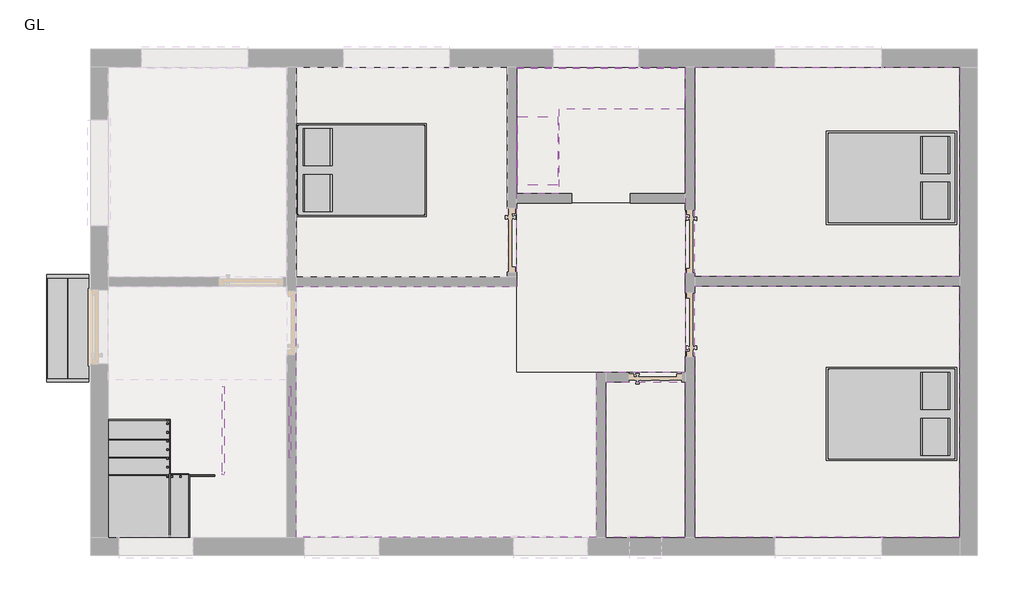
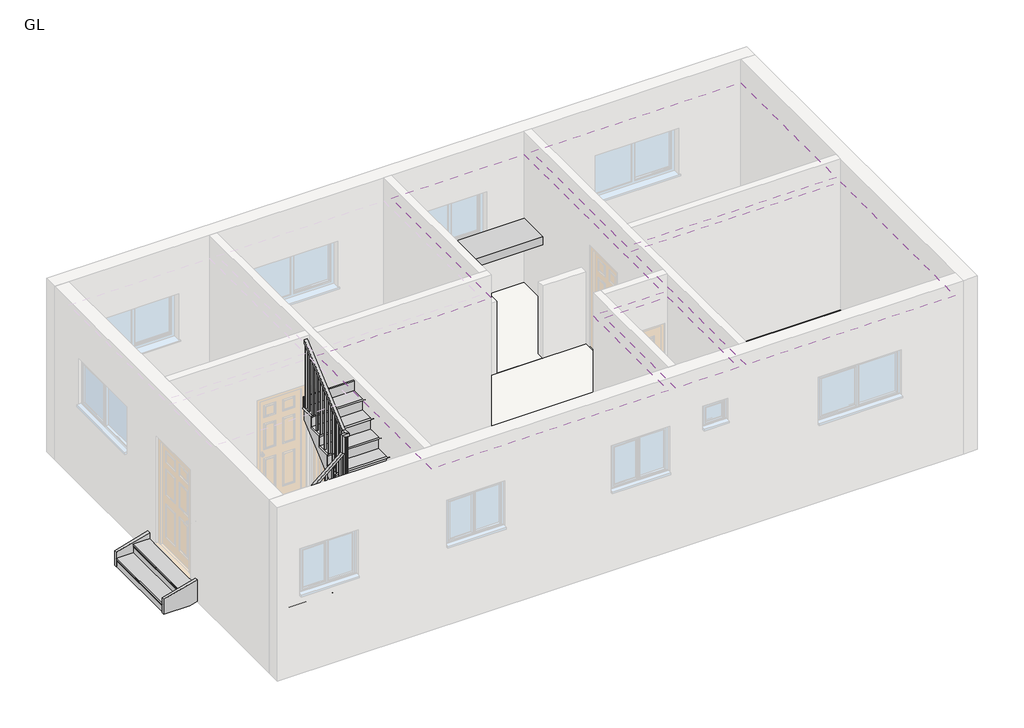
# One storey, part 2 of 2: 7 members, 5 slabs, 4 coverings, 3 furniture elements, 2 proxies, 2 stair flights, 1 railing.
"""IFC4 building model written with IfcOpenShell, lengths in millimetres."""

from ifc_helpers import new_model, si_unit, frame, origin, place, context, project, spatial, polyline, outline, extrude, faceted_brep, transform, mapped, element, save
from components import proxy_0915_x_500_mm_892363c5, furniture_bed_1_1346x1880x355mm_double_93dec6ea, wood_steps_w_30mm_tread_25mm_nosing_19mm_riser_e02fc27e, wood_steps_w_50mm_tread_10mm_nosing_13mm_riser_13d2c295

model = new_model("IFC4")

# Units and contexts
model_context = context("Model", 3, world=origin())
ifc_project = project(units=[si_unit("LENGTHUNIT", "METRE", prefix="MILLI")], contexts=[model_context])

# Site, building, storey
site = spatial("IfcSite", under=ifc_project)
building = spatial("IfcBuilding", under=site)
storey = spatial("IfcBuildingStorey", under=building, Name="GL", Elevation=0.0)

# Proxies
placement = place(None, origin())
proxy_0915_x_500_mm_shape = proxy_0915_x_500_mm_892363c5(model_context)
element("IfcBuildingElementProxy", 1, Name="0915 x 500 mm", ObjectType="0915 x 500 mm", at=placement, inside=storey, context=model_context, shape_type="MappedRepresentation", body=[
    mapped(proxy_0915_x_500_mm_shape, transform((1909.0522582, 5351.5962501, 467.868), x_axis=(0.0, 1.0, 0.0), y_axis=(-1.0, 0.0, 0.0), z_axis=(0.0, 0.0, 1.0))),
])
element("IfcBuildingElementProxy", 2, Name="Generic Models 1 : Generic Models 1", ObjectType="Generic Models 1 : Generic Models 1", at=placement, inside=storey, context=model_context, shape_type="SweptSolid", body=[
    extrude(outline(polyline([(2213.8522582, 4735.0444495), (1604.2522582, 4735.0444495), (1604.2522582, 6545.3962501), (4029.9522582, 6545.3962501), (4029.9522582, 5954.2444495), (2213.8522582, 5954.2444495), (2213.8522582, 4735.0444495)])), frame((0.0, 0.0, 1219.2), z_axis=(0.0, 0.0, 1.0), x_axis=(1.0, 0.0, 0.0)), (0.0, 0.0, 1.0), 152.4),
])

# Coverings
element("IfcCovering", 3, ObjectType="Plain", at=placement, inside=storey, context=model_context, shape_type="SweptSolid", body=[
    extrude(outline(polyline([(1604.2522582, 6562.8522428), (4033.9673421, 6562.8522428), (4033.9673421, 2153.4122428), (2751.2673421, 2153.4122428), (2751.2673421, -234.1877572), (-1580.4996772, -234.1877572), (-1580.4996772, 3389.7573971), (1604.2522582, 3389.7573971), (1604.2522582, 6562.8522428)])), frame((0.0, 0.0, 2600.0), z_axis=(0.0, 0.0, 1.0), x_axis=(1.0, 0.0, 0.0)), (0.0, 0.0, 1.0), 57.0),
])
element("IfcCovering", 4, ObjectType="Plain", at=placement, inside=storey, context=model_context, shape_type="SweptSolid", body=[
    extrude(outline(polyline([(4171.1273421, 6562.8522428), (7994.8922582, 6562.8522428), (7994.8922582, 3534.6060854), (4171.1273421, 3534.6060854), (4171.1273421, 6562.8522428)])), frame((0.0, 0.0, 2600.0), z_axis=(0.0, 0.0, 1.0), x_axis=(1.0, 0.0, 0.0)), (0.0, 0.0, 1.0), 57.0),
])
element("IfcCovering", 5, ObjectType="Plain", at=placement, inside=storey, context=model_context, shape_type="SweptSolid", body=[
    extrude(outline(polyline([(4171.1273421, 3397.4460854), (7994.8922582, 3397.4460854), (7994.8922582, -234.1877572), (4171.1273421, -234.1877572), (4171.1273421, 3397.4460854)])), frame((0.0, 0.0, 2600.0), z_axis=(0.0, 0.0, 1.0), x_axis=(1.0, 0.0, 0.0)), (0.0, 0.0, 1.0), 57.0),
])
element("IfcCovering", 6, ObjectType="Plain", at=placement, inside=storey, context=model_context, shape_type="SweptSolid", body=[
    extrude(outline(polyline([(4033.9673421, 2016.2522428), (4033.9673421, -234.1877572), (2888.4273421, -234.1877572), (2888.4273421, 2016.2522428), (4033.9673421, 2016.2522428)])), frame((0.0, 0.0, 2600.0), z_axis=(0.0, 0.0, 1.0), x_axis=(1.0, 0.0, 0.0)), (0.0, 0.0, 1.0), 57.0),
])

# Furniture
furniture_bed_1_1346x1880x355mm_double_shape = furniture_bed_1_1346x1880x355mm_double_93dec6ea(model_context)
element("IfcFurniture", 7, ObjectType="Furniture_Bed_1 : 1346x1880x355mm-Double", at=placement, inside=storey, context=model_context, shape_type="MappedRepresentation", body=[
    mapped(furniture_bed_1_1346x1880x355mm_double_shape, transform((7249.2052658, 1890.4847018, 124.968), x_axis=(0.0, -1.0, 0.0), y_axis=(1.0, 0.0, 0.0), z_axis=(0.0, 0.0, 1.0))),
])
element("IfcFurniture", 8, ObjectType="Furniture_Bed_1 : 1346x1880x355mm-Double", at=placement, inside=storey, context=model_context, shape_type="MappedRepresentation", body=[
    mapped(furniture_bed_1_1346x1880x355mm_double_shape, transform((7249.2052658, 5301.0698561, 124.968), x_axis=(0.0, -1.0, 0.0), y_axis=(1.0, 0.0, 0.0), z_axis=(0.0, 0.0, 1.0))),
])
element("IfcFurniture", 9, ObjectType="Furniture_Bed_1 : 1346x1880x355mm-Double", at=placement, inside=storey, context=model_context, shape_type="MappedRepresentation", body=[
    mapped(furniture_bed_1_1346x1880x355mm_double_shape, transform((-874.9291854, 4735.0444495, 124.968), x_axis=(0.0, 1.0, 0.0), y_axis=(-1.0, 0.0, 0.0), z_axis=(0.0, 0.0, 1.0))),
])

# Members
element("IfcMember", 10, ObjectType="Stringer-50mm_Width", at=placement, inside=storey, context=model_context, shape_type="SweptSolid", body=[
    extrude(outline(polyline([(-19.9608904, -5182.6277418), (-304.8, -5182.6277418), (-304.8, -4709.8631575), (-267.1702607, -4573.0277418), (147.6791096, -4573.0277418), (-19.9608904, -5182.6277418)])), frame((0.0, 3514.2173971, 0.0), z_axis=(0.0, 1.0, 0.0), x_axis=(0.0, 0.0, 1.0)), (0.0, 0.0, 1.0), 50.0),
])
element("IfcMember", 11, ObjectType="Stringer-50mm_Width", at=placement, inside=storey, context=model_context, shape_type="SweptSolid", body=[
    extrude(outline(polyline([(-19.9608904, -5182.6277418), (-304.8, -5182.6277418), (-304.8, -4709.8631575), (-267.1702607, -4573.0277418), (147.6791096, -4573.0277418), (-19.9608904, -5182.6277418)])), frame((0.0, 2010.6912809, 0.0), z_axis=(0.0, 1.0, 0.0), x_axis=(0.0, 0.0, 1.0)), (0.0, 0.0, 1.0), 50.0),
])
element("IfcMember", 12, ObjectType="Stringer-50mm_Width", at=placement, inside=storey, context=model_context, shape_type="Brep", body=[
    faceted_brep([(-3412.2477418, 1428.6922428, 0.0), (-3412.2477418, 1164.46764, 0.0), (-3437.2477418, 1164.46764, 0.0), (-3437.2477418, 1428.6922428, 0.0), (-3412.2477418, 1428.6922428, 168.645103), (-3412.2477418, 1406.4448629, 187.7142857), (-3412.2477418, 1137.5414829, 187.7142857), (-3412.2477418, 1137.5414829, 405.4285714), (-3412.2477418, 883.5414829, 405.4285714), (-3412.2477418, 883.5414829, 623.1428571), (-3412.2477418, 673.5414829, 623.1428571), (-3412.2477418, 673.5414829, 420.793849), (-3412.2477418, 883.5414829, 240.793849), (-3412.2477418, 1137.5414829, 23.0795633), (-3437.2477418, 673.5414829, 420.793849), (-3437.2477418, 673.5414829, 623.1428571), (-3437.2477418, 1428.6922428, 168.645103), (-3437.2477418, 1137.5414829, 187.7142857), (-3437.2477418, 1406.4448629, 187.7142857), (-3437.2477418, 883.5414829, 623.1428571), (-3437.2477418, 883.5414829, 405.4285714), (-3437.2477418, 1137.5414829, 405.4285714)], [[[0, 1, 2, 3]], [[4, 5, 6, 7, 8, 9, 10, 11, 12, 13, 1, 0]], [[14, 11, 10, 15]], [[11, 14, 2, 1, 13, 12]], [[16, 4, 0, 3]], [[17, 6, 5, 18]], [[18, 16, 3, 2, 14, 15, 19, 20, 21, 17]], [[16, 18, 5, 4]], [[6, 17, 21, 7]], [[7, 21, 20, 8]], [[8, 20, 19, 9]], [[9, 19, 15, 10]]]),
])
element("IfcMember", 13, ObjectType="Stringer-50mm_Width", at=placement, inside=storey, context=model_context, shape_type="Brep", body=[
    faceted_brep([(-3437.2477418, 673.5414829, 618.064712), (-3437.2477418, 673.5414829, 623.1428571), (-3431.2775454, 673.5414829, 623.1428571), (-3437.2477418, 648.5414829, 618.064712), (-3431.2775454, 648.5414829, 623.1428571), (-3437.2477418, 648.5414829, 623.1428571)], [[[0, 1, 2]], [[3, 0, 2, 4]], [[5, 3, 4]], [[0, 3, 5, 1]], [[2, 1, 5, 4]]]),
    faceted_brep([(-2644.3706787, 673.5414829, 1494.0), (-2644.3706787, 673.5414829, 1292.4721338), (-2854.3706787, 673.5414829, 1113.849791), (-3114.2477418, 673.5414829, 892.8028869), (-3368.2477418, 673.5414829, 676.7549104), (-3412.2477418, 673.5414829, 639.3292766), (-3412.2477418, 673.5414829, 840.8571429), (-3368.2477418, 673.5414829, 840.8571429), (-3368.2477418, 673.5414829, 1058.5714286), (-3114.2477418, 673.5414829, 1058.5714286), (-3114.2477418, 673.5414829, 1276.2857143), (-2854.3706787, 673.5414829, 1276.2857143), (-2854.3706787, 673.5414829, 1494.0), (-2644.3706787, 648.5414829, 1292.4721338), (-3412.2477418, 648.5414829, 639.3292766), (-2644.3706787, 648.5414829, 1494.0), (-2854.3706787, 648.5414829, 1494.0), (-2854.3706787, 648.5414829, 1276.2857143), (-3114.2477418, 648.5414829, 1276.2857143), (-3114.2477418, 648.5414829, 1058.5714286), (-3368.2477418, 648.5414829, 1058.5714286), (-3368.2477418, 648.5414829, 840.8571429), (-3412.2477418, 648.5414829, 840.8571429)], [[[0, 1, 2, 3, 4, 5, 6, 7, 8, 9, 10, 11, 12]], [[1, 13, 14, 5, 4, 3, 2]], [[14, 13, 15, 16, 17, 18, 19, 20, 21, 22]], [[13, 1, 0, 15]], [[10, 18, 17, 11]], [[6, 22, 21, 7]], [[22, 6, 5, 14]], [[8, 20, 19, 9]], [[7, 21, 20, 8]], [[18, 10, 9, 19]], [[12, 16, 15, 0]], [[11, 17, 16, 12]]]),
])
element("IfcMember", 14, ObjectType="Stringer-50mm_Width", at=placement, inside=storey, context=model_context, shape_type="Brep", body=[
    faceted_brep([(-2619.3706787, 1948.6214829, 2602.2909918), (-2644.3706787, 1948.6214829, 2602.2909918), (-2644.3706787, 1948.6214829, 2800.2857143), (-2619.3706787, 1948.6214829, 2800.2857143), (-2644.3706787, 1733.5414829, 2417.9367061), (-2644.3706787, 1479.5414829, 2200.2224204), (-2644.3706787, 1225.5414829, 1982.5081347), (-2644.3706787, 971.5414829, 1764.793849), (-2644.3706787, 717.5414829, 1547.0795633), (-2644.3706787, 673.5414829, 1509.3652775), (-2644.3706787, 673.5414829, 1711.7142857), (-2644.3706787, 717.5414829, 1711.7142857), (-2644.3706787, 717.5414829, 1929.4285714), (-2644.3706787, 971.5414829, 1929.4285714), (-2644.3706787, 971.5414829, 2147.1428571), (-2644.3706787, 1225.5414829, 2147.1428571), (-2644.3706787, 1225.5414829, 2364.8571429), (-2644.3706787, 1479.5414829, 2364.8571429), (-2644.3706787, 1479.5414829, 2582.5714286), (-2644.3706787, 1733.5414829, 2582.5714286), (-2644.3706787, 1733.5414829, 2800.2857143), (-2619.3706787, 673.5414829, 1509.3652775), (-2619.3706787, 1733.5414829, 2800.2857143), (-2619.3706787, 1733.5414829, 2582.5714286), (-2619.3706787, 1479.5414829, 2582.5714286), (-2619.3706787, 1479.5414829, 2364.8571429), (-2619.3706787, 1225.5414829, 2364.8571429), (-2619.3706787, 1225.5414829, 2147.1428571), (-2619.3706787, 971.5414829, 2147.1428571), (-2619.3706787, 971.5414829, 1929.4285714), (-2619.3706787, 717.5414829, 1929.4285714), (-2619.3706787, 717.5414829, 1711.7142857), (-2619.3706787, 673.5414829, 1711.7142857)], [[[0, 1, 2, 3]], [[2, 1, 4, 5, 6, 7, 8, 9, 10, 11, 12, 13, 14, 15, 16, 17, 18, 19, 20]], [[1, 0, 21, 9, 8, 7, 6, 5, 4]], [[0, 3, 22, 23, 24, 25, 26, 27, 28, 29, 30, 31, 32, 21]], [[10, 32, 31, 11]], [[32, 10, 9, 21]], [[12, 30, 29, 13]], [[11, 31, 30, 12]], [[14, 28, 27, 15]], [[13, 29, 28, 14]], [[16, 26, 25, 17]], [[15, 27, 26, 16]], [[18, 24, 23, 19]], [[17, 25, 24, 18]], [[20, 22, 3, 2]], [[19, 23, 22, 20]]]),
    faceted_brep([(-2644.3706787, 648.5414829, 1487.9367061), (-2644.3706787, 648.5414829, 1494.0), (-2644.3706787, 655.6153258, 1494.0), (-2619.3706787, 648.5414829, 1487.9367061), (-2619.3706787, 655.6153258, 1494.0), (-2619.3706787, 648.5414829, 1494.0)], [[[0, 1, 2]], [[3, 0, 2, 4]], [[5, 3, 4]], [[0, 3, 5, 1]], [[2, 1, 5, 4]]]),
])
element("IfcMember", 15, ObjectType="Stringer-50mm_Width", at=placement, inside=storey, context=model_context, shape_type="SweptSolid", body=[
    extrude(outline(polyline([(1472.6922428, 130.9308173), (1472.6922428, 0.0), (1164.46764, 0.0), (879.101533, 244.5995203), (1340.0787559, 244.5995203), (1472.6922428, 130.9308173)])), frame((-4364.3477418, 0.0, 0.0), z_axis=(1.0, 0.0, 0.0), x_axis=(0.0, 1.0, 0.0)), (0.0, 0.0, 1.0), 25.0),
])
element("IfcMember", 16, ObjectType="Stringer-50mm_Width", at=placement, inside=storey, context=model_context, shape_type="SweptSolid", body=[
    extrude(outline(polyline([(916.9489336, 2113.1235692), (1948.6214829, 2997.4143257), (1948.6214829, 2602.2909918), (1377.9261565, 2113.1235692), (916.9489336, 2113.1235692)])), frame((-1679.5596772, 0.0, 0.0), z_axis=(1.0, 0.0, 0.0), x_axis=(0.0, 1.0, 0.0)), (0.0, 0.0, 1.0), 25.0),
])

# Railing
element("IfcRailing", 17, ObjectType="1100mm", at=placement, inside=storey, context=model_context, shape_type="SolidModel", body=[
    faceted_brep([(-3412.6477418, 1472.6922428, 1317.7142857), (-3412.6477418, 1472.6922428, 1253.1392706), (-3462.6477418, 1472.6922428, 1253.1392706), (-3462.6477418, 1472.6922428, 1317.7142857), (-3412.6477418, 748.1414829, 1909.8868484), (-3412.6477418, 698.1414829, 1886.1766419), (-3462.6477418, 698.1414829, 1886.1766419), (-3462.6477418, 748.1414829, 1909.8868484), (-3412.6477418, 748.1414829, 2252.0248894), (-3412.6477418, 698.1414829, 2202.0248894), (-3462.6477418, 698.1414829, 2202.0248894), (-3462.6477418, 748.1414829, 2252.0248894), (-3412.6477418, 673.1414829, 2252.0248894), (-3412.6477418, 673.1414829, 2202.0248894), (-3462.6477418, 623.1414829, 2202.0248894), (-3462.6477418, 623.1414829, 2252.0248894), (-3337.6477418, 673.1414829, 2252.0248894), (-3319.2592946, 673.1414829, 2202.0248894), (-3319.2592946, 623.1414829, 2202.0248894), (-3337.6477418, 623.1414829, 2252.0248894), (-2718.9706787, 673.1414829, 2778.2608249), (-2668.9706787, 673.1414829, 2755.1490611), (-2668.9706787, 623.1414829, 2755.1490611), (-2718.9706787, 623.1414829, 2778.2608249), (-2718.9706787, 673.1414829, 3123.1166762), (-2668.9706787, 673.1414829, 3073.1166762), (-2668.9706787, 623.1414829, 3073.1166762), (-2718.9706787, 623.1414829, 3123.1166762), (-2643.9706787, 673.1414829, 3123.1166762), (-2643.9706787, 673.1414829, 3073.1166762), (-2593.9706787, 623.1414829, 3073.1166762), (-2593.9706787, 623.1414829, 3123.1166762), (-2643.9706787, 748.1414829, 3123.1166762), (-2643.9706787, 766.581663, 3073.1166762), (-2593.9706787, 766.581663, 3073.1166762), (-2593.9706787, 748.1414829, 3123.1166762), (-2643.9706787, 1948.6214829, 4148.0), (-2593.9706787, 1948.6214829, 4148.0), (-2593.9706787, 1948.6214829, 4082.257103), (-2643.9706787, 1948.6214829, 4082.257103)], [[[0, 1, 2, 3]], [[1, 0, 4, 5]], [[2, 1, 5, 6]], [[3, 2, 6, 7]], [[0, 3, 7, 4]], [[5, 4, 8, 9]], [[6, 5, 9, 10]], [[7, 6, 10, 11]], [[4, 7, 11, 8]], [[9, 8, 12, 13]], [[10, 9, 13, 14]], [[11, 10, 14, 15]], [[8, 11, 15, 12]], [[13, 12, 16, 17]], [[14, 13, 17, 18]], [[15, 14, 18, 19]], [[12, 15, 19, 16]], [[17, 16, 20, 21]], [[18, 17, 21, 22]], [[19, 18, 22, 23]], [[16, 19, 23, 20]], [[21, 20, 24, 25]], [[22, 21, 25, 26]], [[23, 22, 26, 27]], [[20, 23, 27, 24]], [[25, 24, 28, 29]], [[26, 25, 29, 30]], [[27, 26, 30, 31]], [[24, 27, 31, 28]], [[29, 28, 32, 33]], [[30, 29, 33, 34]], [[31, 30, 34, 35]], [[28, 31, 35, 32]], [[36, 37, 38, 39]], [[33, 32, 36, 39]], [[34, 33, 39, 38]], [[35, 34, 38, 37]], [[32, 35, 37, 36]]]),
    extrude(outline(polyline([(1823.1414829, 3975.1313204), (1848.1414829, 3996.474519), (1848.1414829, 2830.2857143), (1823.1414829, 2830.2857143), (1823.1414829, 3975.1313204)])), frame((-2631.4706787, 0.0, 0.0), z_axis=(1.0, 0.0, 0.0), x_axis=(0.0, 1.0, 0.0)), (0.0, 0.0, 1.0), 25.0),
    extrude(outline(polyline([(1698.1414829, 3868.4153272), (1723.1414829, 3889.7585258), (1723.1414829, 2830.2857143), (1698.1414829, 2830.2857143), (1698.1414829, 3868.4153272)])), frame((-2631.4706787, 0.0, 0.0), z_axis=(1.0, 0.0, 0.0), x_axis=(0.0, 1.0, 0.0)), (0.0, 0.0, 1.0), 25.0),
    extrude(outline(polyline([(1573.1414829, 3761.699334), (1598.1414829, 3783.0425327), (1598.1414829, 2612.5714286), (1573.1414829, 2612.5714286), (1573.1414829, 3761.699334)])), frame((-2631.4706787, 0.0, 0.0), z_axis=(1.0, 0.0, 0.0), x_axis=(0.0, 1.0, 0.0)), (0.0, 0.0, 1.0), 25.0),
    extrude(outline(polyline([(1448.1414829, 3654.9833409), (1473.1414829, 3676.3265395), (1473.1414829, 2612.5714286), (1448.1414829, 2612.5714286), (1448.1414829, 3654.9833409)])), frame((-2631.4706787, 0.0, 0.0), z_axis=(1.0, 0.0, 0.0), x_axis=(0.0, 1.0, 0.0)), (0.0, 0.0, 1.0), 25.0),
    extrude(outline(polyline([(1323.1414829, 3548.2673477), (1348.1414829, 3569.6105463), (1348.1414829, 2394.8571429), (1323.1414829, 2394.8571429), (1323.1414829, 3548.2673477)])), frame((-2631.4706787, 0.0, 0.0), z_axis=(1.0, 0.0, 0.0), x_axis=(0.0, 1.0, 0.0)), (0.0, 0.0, 1.0), 25.0),
    extrude(outline(polyline([(1198.1414829, 3441.5513545), (1223.1414829, 3462.8945532), (1223.1414829, 2394.8571429), (1198.1414829, 2394.8571429), (1198.1414829, 3441.5513545)])), frame((-2631.4706787, 0.0, 0.0), z_axis=(1.0, 0.0, 0.0), x_axis=(0.0, 1.0, 0.0)), (0.0, 0.0, 1.0), 25.0),
    extrude(outline(polyline([(1073.1414829, 3334.8353614), (1098.1414829, 3356.17856), (1098.1414829, 2177.1428571), (1073.1414829, 2177.1428571), (1073.1414829, 3334.8353614)])), frame((-2631.4706787, 0.0, 0.0), z_axis=(1.0, 0.0, 0.0), x_axis=(0.0, 1.0, 0.0)), (0.0, 0.0, 1.0), 25.0),
    extrude(outline(polyline([(948.1414829, 3228.1193682), (973.1414829, 3249.4625668), (973.1414829, 2177.1428571), (948.1414829, 2177.1428571), (948.1414829, 3228.1193682)])), frame((-2631.4706787, 0.0, 0.0), z_axis=(1.0, 0.0, 0.0), x_axis=(0.0, 1.0, 0.0)), (0.0, 0.0, 1.0), 25.0),
    extrude(outline(polyline([(823.1414829, 3121.403375), (848.1414829, 3142.7465736), (848.1414829, 1959.4285714), (823.1414829, 1959.4285714), (823.1414829, 3121.403375)])), frame((-2631.4706787, 0.0, 0.0), z_axis=(1.0, 0.0, 0.0), x_axis=(0.0, 1.0, 0.0)), (0.0, 0.0, 1.0), 25.0),
    extrude(outline(polyline([(-2631.4706787, 698.1414829), (-2631.4706787, 723.1414829), (-2606.4706787, 723.1414829), (-2606.4706787, 698.1414829), (-2631.4706787, 698.1414829)])), frame((0.0, 0.0, 1959.4285714), z_axis=(0.0, 0.0, 1.0), x_axis=(1.0, 0.0, 0.0)), (0.0, 0.0, 1.0), 1113.6881047),
    extrude(outline(polyline([(-2637.6477418, 660.6414829), (-2612.6477418, 660.6414829), (-2612.6477418, 635.6414829), (-2637.6477418, 635.6414829), (-2637.6477418, 660.6414829)])), frame((0.0, 0.0, 1741.7142857), z_axis=(0.0, 0.0, 1.0), x_axis=(1.0, 0.0, 0.0)), (0.0, 0.0, 1.0), 1331.4023904),
    extrude(outline(polyline([(1524.0, -2762.6477418), (1524.0, -2737.6477418), (2696.7335472, -2737.6477418), (2675.4689826, -2762.6477418), (1524.0, -2762.6477418)])), frame((0.0, 635.6414829, 0.0), z_axis=(0.0, 1.0, 0.0), x_axis=(0.0, 0.0, 1.0)), (0.0, 0.0, 1.0), 25.0),
    extrude(outline(polyline([(1524.0, -2887.6477418), (1524.0, -2862.6477418), (2590.4107241, -2862.6477418), (2569.1461595, -2887.6477418), (1524.0, -2887.6477418)])), frame((0.0, 635.6414829, 0.0), z_axis=(0.0, 1.0, 0.0), x_axis=(0.0, 0.0, 1.0)), (0.0, 0.0, 1.0), 25.0),
    extrude(outline(polyline([(1306.2857143, -3012.6477418), (1306.2857143, -2987.6477418), (2484.0879011, -2987.6477418), (2462.8233364, -3012.6477418), (1306.2857143, -3012.6477418)])), frame((0.0, 635.6414829, 0.0), z_axis=(0.0, 1.0, 0.0), x_axis=(0.0, 0.0, 1.0)), (0.0, 0.0, 1.0), 25.0),
    extrude(outline(polyline([(1306.2857143, -3137.6477418), (1306.2857143, -3112.6477418), (2377.765078, -3112.6477418), (2356.5005133, -3137.6477418), (1306.2857143, -3137.6477418)])), frame((0.0, 635.6414829, 0.0), z_axis=(0.0, 1.0, 0.0), x_axis=(0.0, 0.0, 1.0)), (0.0, 0.0, 1.0), 25.0),
    extrude(outline(polyline([(1088.5714286, -3262.6477418), (1088.5714286, -3237.6477418), (2271.4422549, -3237.6477418), (2250.1776903, -3262.6477418), (1088.5714286, -3262.6477418)])), frame((0.0, 635.6414829, 0.0), z_axis=(0.0, 1.0, 0.0), x_axis=(0.0, 0.0, 1.0)), (0.0, 0.0, 1.0), 25.0),
    extrude(outline(polyline([(-3387.6477418, 660.6414829), (-3362.6477418, 660.6414829), (-3362.6477418, 635.6414829), (-3387.6477418, 635.6414829), (-3387.6477418, 660.6414829)])), frame((0.0, 0.0, 1088.5714286), z_axis=(0.0, 0.0, 1.0), x_axis=(1.0, 0.0, 0.0)), (0.0, 0.0, 1.0), 1113.4534608),
    extrude(outline(polyline([(-3425.1477418, 672.6922428), (-3425.1477418, 647.6922428), (-3450.1477418, 647.6922428), (-3450.1477418, 672.6922428), (-3425.1477418, 672.6922428)])), frame((0.0, 0.0, 870.8571429), z_axis=(0.0, 0.0, 1.0), x_axis=(1.0, 0.0, 0.0)), (0.0, 0.0, 1.0), 1331.1677465),
    extrude(outline(polyline([(797.6922428, 653.1428571), (772.6922428, 653.1428571), (772.6922428, 1825.2465912), (797.6922428, 1804.8141869), (797.6922428, 653.1428571)])), frame((-3450.1477418, 0.0, 0.0), z_axis=(1.0, 0.0, 0.0), x_axis=(0.0, 1.0, 0.0)), (0.0, 0.0, 1.0), 25.0),
    extrude(outline(polyline([(922.6922428, 653.1428571), (897.6922428, 653.1428571), (897.6922428, 1723.0845696), (922.6922428, 1702.6521653), (922.6922428, 653.1428571)])), frame((-3450.1477418, 0.0, 0.0), z_axis=(1.0, 0.0, 0.0), x_axis=(0.0, 1.0, 0.0)), (0.0, 0.0, 1.0), 25.0),
    extrude(outline(polyline([(1047.6922428, 435.4285714), (1022.6922428, 435.4285714), (1022.6922428, 1620.9225481), (1047.6922428, 1600.4901438), (1047.6922428, 435.4285714)])), frame((-3450.1477418, 0.0, 0.0), z_axis=(1.0, 0.0, 0.0), x_axis=(0.0, 1.0, 0.0)), (0.0, 0.0, 1.0), 25.0),
    extrude(outline(polyline([(1172.6922428, 435.4285714), (1147.6922428, 435.4285714), (1147.6922428, 1518.7605266), (1172.6922428, 1498.3281222), (1172.6922428, 435.4285714)])), frame((-3450.1477418, 0.0, 0.0), z_axis=(1.0, 0.0, 0.0), x_axis=(0.0, 1.0, 0.0)), (0.0, 0.0, 1.0), 25.0),
    extrude(outline(polyline([(1297.6922428, 217.7142857), (1272.6922428, 217.7142857), (1272.6922428, 1416.598505), (1297.6922428, 1396.1661007), (1297.6922428, 217.7142857)])), frame((-3450.1477418, 0.0, 0.0), z_axis=(1.0, 0.0, 0.0), x_axis=(0.0, 1.0, 0.0)), (0.0, 0.0, 1.0), 25.0),
    extrude(outline(polyline([(1422.6922428, 217.7142857), (1397.6922428, 217.7142857), (1397.6922428, 1314.4364835), (1422.6922428, 1294.0040792), (1422.6922428, 217.7142857)])), frame((-3450.1477418, 0.0, 0.0), z_axis=(1.0, 0.0, 0.0), x_axis=(0.0, 1.0, 0.0)), (0.0, 0.0, 1.0), 25.0),
    extrude(outline(polyline([(-2631.4706787, 660.6414829), (-2606.4706787, 660.6414829), (-2606.4706787, 635.6414829), (-2631.4706787, 635.6414829), (-2631.4706787, 660.6414829)])), frame((0.0, 0.0, 1741.7142857), z_axis=(0.0, 0.0, 1.0), x_axis=(1.0, 0.0, 0.0)), (0.0, 0.0, 1.0), 1331.4023904),
    extrude(outline(polyline([(-3425.1477418, 660.6414829), (-3425.1477418, 635.6414829), (-3450.1477418, 635.6414829), (-3450.1477418, 660.6414829), (-3425.1477418, 660.6414829)])), frame((0.0, 0.0, 870.8571429), z_axis=(0.0, 0.0, 1.0), x_axis=(1.0, 0.0, 0.0)), (0.0, 0.0, 1.0), 1331.1677465),
    extrude(outline(polyline([(1923.6214829, 4060.7175396), (1948.6214829, 4082.146111), (1948.6214829, 2830.2857143), (1923.6214829, 2830.2857143), (1923.6214829, 4060.7175396)])), frame((-2631.4706787, 0.0, 0.0), z_axis=(1.0, 0.0, 0.0), x_axis=(0.0, 1.0, 0.0)), (0.0, 0.0, 1.0), 25.0),
    extrude(outline(polyline([(1472.6922428, 217.7142857), (1447.6922428, 217.7142857), (1447.6922428, 1273.5716749), (1472.6922428, 1253.1392706), (1472.6922428, 217.7142857)])), frame((-3450.1477418, 0.0, 0.0), z_axis=(1.0, 0.0, 0.0), x_axis=(0.0, 1.0, 0.0)), (0.0, 0.0, 1.0), 25.0),
])

# Slabs
element("IfcSlab", 18, ObjectType="BEDROOM FLOOR", at=placement, inside=storey, context=model_context, shape_type="SweptSolid", body=[
    extrude(outline(polyline([(1604.2522582, 6562.8522428), (1604.2522582, 3526.9173971), (-1580.4996772, 3526.9173971), (-1580.4996772, 6562.8522428), (1604.2522582, 6562.8522428)])), frame((0.0, 0.0, -24.9936), z_axis=(0.0, 0.0, 1.0), x_axis=(1.0, 0.0, 0.0)), (0.0, 0.0, 1.0), 149.9616),
    extrude(outline(polyline([(4033.9673421, 3534.6060854), (4033.9673421, 6562.8522428), (7994.8922582, 6562.8522428), (7994.8922582, 3534.6060854), (4033.9673421, 3534.6060854)])), frame((0.0, 0.0, -24.9936), z_axis=(0.0, 0.0, 1.0), x_axis=(1.0, 0.0, 0.0)), (0.0, 0.0, 1.0), 149.9616),
])
element("IfcSlab", 19, ObjectType="BEDROOM FLOOR", at=placement, inside=storey, context=model_context, shape_type="SweptSolid", body=[
    extrude(outline(polyline([(4033.9673421, -234.1877572), (4033.9673421, 3526.9173971), (7994.8922582, 3526.9173971), (7994.8922582, -234.1877572), (4033.9673421, -234.1877572)])), frame((0.0, 0.0, -24.9936), z_axis=(0.0, 0.0, 1.0), x_axis=(1.0, 0.0, 0.0)), (0.0, 0.0, 1.0), 149.9616),
])
element("IfcSlab", 20, ObjectType="DINING FLOOR", at=placement, inside=storey, context=model_context, shape_type="Brep", body=[
    faceted_brep([(1604.2522582, 2153.4122428, -24.9936), (1604.2522582, 4597.8844495, -24.9936), (4033.9673421, 4597.8844495, -24.9936), (4033.9673421, 2153.4122428, -24.9936), (2751.2673421, 2153.4122428, -24.9936), (1604.2522582, 2153.4122428, 124.968), (2751.2673421, 2153.4122428, 124.968), (4033.9673421, 2153.4122428, 124.968), (4033.9673421, 4597.8844495, 124.968), (1604.2522582, 4597.8844495, 124.968)], [[[0, 1, 2, 3, 4]], [[5, 6, 7, 8, 9]], [[1, 0, 5, 9]], [[2, 1, 9, 8]], [[3, 2, 8, 7]], [[0, 4, 3, 7, 6, 5]]]),
])
element("IfcSlab", 21, ObjectType="KITCHEN FLOOR", at=placement, inside=storey, context=model_context, shape_type="SweptSolid", body=[
    extrude(outline(polyline([(4029.9522582, 6562.8522428), (4029.9522582, 4597.8844495), (1604.2522582, 4597.8844495), (1604.2522582, 6562.8522428), (4029.9522582, 6562.8522428)])), frame((0.0, 0.0, -24.9936), z_axis=(0.0, 0.0, 1.0), x_axis=(1.0, 0.0, 0.0)), (0.0, 0.0, 1.0), 149.9616),
])
element("IfcSlab", 22, ObjectType="TOILET FLOOR", at=placement, inside=storey, context=model_context, shape_type="SweptSolid", body=[
    extrude(outline(polyline([(2751.2673421, -234.1877572), (2751.2673421, 2153.4122428), (4033.9673421, 2153.4122428), (4033.9673421, -234.1877572), (2751.2673421, -234.1877572)])), frame((0.0, 0.0, -24.9936), z_axis=(0.0, 0.0, 1.0), x_axis=(1.0, 0.0, 0.0)), (0.0, 0.0, 1.0), 149.9616),
])

# Stair flights
wood_steps_w_30mm_tread_25mm_nosing_19mm_riser_shape = wood_steps_w_30mm_tread_25mm_nosing_19mm_riser_e02fc27e(model_context)
element("IfcStairFlight", 23, ObjectType="Wood_Steps_w-30mm_Tread-25mm_Nosing-19mm_Riser", at=placement, inside=storey, context=model_context, shape_type="MappedRepresentation", body=[
    mapped(wood_steps_w_30mm_tread_25mm_nosing_19mm_riser_shape, transform((0.0, 0.0, 0.0), x_axis=(1.0, 0.0, 0.0), y_axis=(0.0, 1.0, 0.0), z_axis=(0.0, 0.0, 1.0))),
])
wood_steps_w_50mm_tread_10mm_nosing_13mm_riser_shape = wood_steps_w_50mm_tread_10mm_nosing_13mm_riser_13d2c295(model_context)
element("IfcStairFlight", 24, ObjectType="Wood_Steps_w-50mm_Tread-10mm_Nosing-13mm_Riser", at=placement, inside=storey, context=model_context, shape_type="MappedRepresentation", body=[
    mapped(wood_steps_w_50mm_tread_10mm_nosing_13mm_riser_shape, transform((0.0, 0.0, 0.0), x_axis=(1.0, 0.0, 0.0), y_axis=(0.0, 1.0, 0.0), z_axis=(0.0, 0.0, 1.0))),
])

save(model, "model.ifc")

# Revit data of these elements
# Type "0915 x 500 mm"
#   Profundidad = 500 mm
#   Anchura = 915 mm
#   Máscara [instance default] = yes
#   Quemador = Metal - Cromo
#   Cocina encimera = Metal - Acero, Pulido
#   Default Elevation = 0
# Type "Plain"
#   Keynote = "K40"
#   built-in parameter 1002203 = 1 (stored number, unit not read)
#   built-in parameter 1002202 = 1 (stored number, unit not read)
#   Layers, outside or top first: 45 mm "Metal Stud Layer" (function 1); 12 mm "Gypsum Wall Board" (function 1)
# Type "Furniture_Bed_1 : 1346x1880x355mm-Double"
#   Keynote = "N"
#   Length = 1880 mm
#   Width = 1346 mm
#   Material Frame = Wood - Birch
#   Material Mattress = Textile - White
#   Default Elevation = 0
# Type "1100mm"
#   built-in parameter 1008612 = 0.019685 (stored number, unit not read)
#   built-in parameter 1008611 = 0.019685 (stored number, unit not read)
#   built-in parameter 1008609 = 0.902231 (stored number, unit not read)
#   built-in parameter 1008604 = 0.19685 (stored number, unit not read)
#   built-in parameter 1008603 = 0.164042 (stored number, unit not read)
#   Railing Height = 1100 mm
#   built-in parameter 1008630 = 2
#   built-in parameter 1008610 = 2
#   built-in parameter 1008608 = 1
#   built-in parameter 1008618 = Baluster_Square : 25mm
# Type "BEDROOM FLOOR"
#   Function = 0
#   Layers, outside or top first: 21.946 mm "Wood Sheathing, Chipboard" (function 5); 128.016 mm "Structure, Timber Joist/Rafter Layer" (function 1)
# Type "DINING FLOOR"
#   Function = 0
#   Layers, outside or top first: 21.946 mm "Wood Sheathing, Chipboard" (function 5); 128.016 mm "Structure, Timber Joist/Rafter Layer" (function 1)
# Type "KITCHEN FLOOR"
#   Function = 0
#   Layers, outside or top first: 21.946 mm "Wood Sheathing, Chipboard" (function 5); 128.016 mm "Structure, Timber Joist/Rafter Layer" (function 1)
# Type "TOILET FLOOR"
#   Function = 0
#   Layers, outside or top first: 21.946 mm "Wood Sheathing, Chipboard" (function 5); 128.016 mm "Structure, Timber Joist/Rafter Layer" (function 1)
# Element 1 (IfcBuildingElementProxy, "0915 x 500 mm")
#   Máscara = yes
#   Phase Created = New Construction
#   Materials on its faces: "Metal - Cromo", "Metal - Acero, Pulido"
# Element 2 (IfcBuildingElementProxy, "Generic Models 1 : Generic Models 1")
#   Phase Created = New Construction
# Elements 3, 4, 5, 6 (IfcCovering, "Plain")
#   Height Offset From Level = 2600 mm
#   Phase Created = New Construction
#   Materials on its faces: "Gypsum Wall Board", "Metal Stud Layer"
# Elements 7, 8, 9 (IfcFurniture, "Furniture_Bed_1 : 1346x1880x355mm-Double")
#   Phase Created = New Construction
#   Materials on its faces: "Wood - Birch", "Textile - White"
# Elements 10, 11 (IfcMember, "Stringer-50mm_Width")
#   Phase Created = New Construction
# Elements 12, 13, 14, 15, 16 (IfcMember, "Stringer-50mm_Width")
#   Phase Created = New Construction
#   Materials on its faces: "Wood"
# Element 17 (IfcRailing, "1100mm")
#   Phase Created = New Construction
# Element 18 (IfcSlab, "BEDROOM FLOOR")
#   Height Offset From Level = 124.968 mm
#   Phase Created = New Construction
#   Materials on its faces: "Structure, Timber Joist/Rafter Layer", "Wood Sheathing, Chipboard"
# Element 19 (IfcSlab, "BEDROOM FLOOR")
#   built-in parameter 1001955 = 3.14159 (stored number, unit not read)
#   Height Offset From Level = 124.968 mm
#   Phase Created = New Construction
#   Materials on its faces: "Structure, Timber Joist/Rafter Layer", "Wood Sheathing, Chipboard"
# Element 20 (IfcSlab, "DINING FLOOR")
#   built-in parameter 1001955 = 3.14159 (stored number, unit not read)
#   Height Offset From Level = 124.968 mm
#   Phase Created = New Construction
#   Materials on its faces: "Structure, Timber Joist/Rafter Layer", "Wood Sheathing, Chipboard"
# Element 21 (IfcSlab, "KITCHEN FLOOR")
#   Height Offset From Level = 124.968 mm
#   Phase Created = New Construction
#   Materials on its faces: "Structure, Timber Joist/Rafter Layer", "Wood Sheathing, Chipboard"
# Element 22 (IfcSlab, "TOILET FLOOR")
#   built-in parameter 1001955 = 3.14159 (stored number, unit not read)
#   Height Offset From Level = 124.968 mm
#   Phase Created = New Construction
#   Materials on its faces: "Structure, Timber Joist/Rafter Layer", "Wood Sheathing, Chipboard"
# Element 23 (IfcStairFlight, "Wood_Steps_w-30mm_Tread-25mm_Nosing-19mm_Riser")
#   Phase Created = New Construction
#   Materials on its faces: "Cherry", "Wood"
# Element 24 (IfcStairFlight, "Wood_Steps_w-50mm_Tread-10mm_Nosing-13mm_Riser")
#   Phase Created = New Construction
#   Materials on its faces: "Oak Flooring"
# Materials
#   "Metal - Cromo": class "Metal", colour RGB 17 17 17, transparency 0
#   "Metal - Acero, Pulido": class "Metal", colour RGB 57 57 57, transparency 0
#   "Metal Stud Layer": class "Metal", colour RGB 127 127 127, transparency 0, Description = "Light gauge steel framing, thermal air layer", Cost = 0
#   "Gypsum Wall Board": class "Generic", colour RGB 249 249 249, transparency 0, Description = "Gypsum Wall Board", Cost = 0
#   "Wood - Birch": class "Wood", colour RGB 224 178 126, transparency 0
#   "Textile - White": class "Fabric", colour RGB 247 247 239, transparency 0
#   "Wood Sheathing, Chipboard": class "Wood", colour RGB 127 127 127, transparency 0, Description = "Particleboard sheathing", Cost = 0
#   "Structure, Timber Joist/Rafter Layer": class "Wood", colour RGB 127 127 127, transparency 0, Description = "Timber framing, thermal airspace", Cost = 0
#   "Wood": class "Wood", colour RGB 212 179 113, transparency 0, Description = "Generic wood", Cost = 0
#   "Cherry": class "Wood", colour RGB 226 177 128, transparency 0, Description = "Prunus Serotina", Cost = 0
#   "Oak Flooring": class "Wood", colour RGB 212 179 113, transparency 0, Description = "Quercus Rubra", Cost = 0
